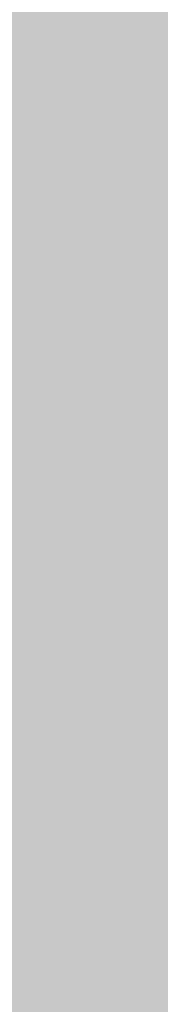
# Model space of a CAD drawing. Units: inches. Extents: x 2083 to 3317, y 1141 to 2115.
# Tile 172 of 256: x 3126.95594 to 3126.95825, y 1263.27402 to 1263.29018. Entities that reach past the tile are written whole.
import ezdxf

# ---------------------------------------------------------------- set-up
doc = ezdxf.new("R2010")
doc.units = ezdxf.units.IN
doc.layers.add('A-ANNO-DIMS', color=2, linetype='Continuous', lineweight=18)
doc.layers.add('A-WALL-PATT', color=251, linetype='Continuous', lineweight=13, true_color=0x636466)
doc.styles.get("Standard").update_dxf_attribs({"font": 'arial.ttf'})
doc.dimstyles.new('ISO-25', dxfattribs={"dimtxt": 12, "dimasz": 12, "dimexe": 1.25, "dimexo": 0.625, "dimtad": 1, "dimlunit": 3, "dimtxsty": 'Standard', "dimcen": 2.5, "dimadec": 0, "dimazin": 0, "dimtfac": 1, "dimtmove": 0, "dimatfit": 3, "dimfxl": 1, "dimarcsym": 0})

# ---------------------------------------------------------------- blocks, each defined once
blk = doc.blocks.new('*D26')
at = {"layer": 'A-ANNO-DIMS', "color": 0, "lineweight": -2, "transparency": 16777216}
for p, q in [((3088.985844, 1274.915092), (3088.985844, 1270.951963)), ((3111.240037, 1274.915092), (3111.240037, 1270.951963)), ((3076.985844, 1272.201963), (2840.262447, 1272.201963)), ((3111.240037, 1272.201963), (3088.985844, 1272.201963)), ((3123.240037, 1272.201963), (3135.240037, 1272.201963))]:
    blk.add_line(p, q, dxfattribs=at)
at = {"layer": 'A-ANNO-DIMS', "color": 0, "transparency": 16777216}
for points in [[(3076.985844, 1274.201963), (3076.985844, 1270.201963), (3088.985844, 1272.201963)], [(3123.240037, 1274.201963), (3123.240037, 1270.201963), (3111.240037, 1272.201963)]]:
    blk.add_solid(points, dxfattribs=at)
at = {"layer": 'Defpoints', "color": 0, "transparency": 16777216}
for p in [(3088.985844, 1275.540092), (3111.240037, 1275.540092), (3088.985844, 1272.201963)]:
    blk.add_point(p, dxfattribs=at)
at = {"layer": 'A-ANNO-DIMS', "color": 0, "transparency": 16777216, "insert": (2952.624146, 1279.031602), "char_height": 12, "attachment_point": 5}
blk.add_mtext('NIGHTSTAND 1\'-10 1/2" TYP.', dxfattribs=at)
blk = doc.blocks.new('*D27')
at = {"layer": 'A-ANNO-DIMS', "color": 0, "lineweight": -2, "transparency": 16777216}
for p, q in [((3114.578165, 1309.794285), (3114.578165, 1321.794285)), ((3111.865037, 1297.794285), (3115.828165, 1297.794285)), ((3114.578165, 1297.794285), (3114.578165, 1275.540092)), ((3111.865037, 1275.540092), (3115.828165, 1275.540092)), ((3114.578165, 1263.540092), (3114.578165, 1140.988591))]:
    blk.add_line(p, q, dxfattribs=at)
at = {"layer": 'A-ANNO-DIMS', "color": 0, "transparency": 16777216}
for points in [[(3112.578165, 1309.794285), (3116.578165, 1309.794285), (3114.578165, 1297.794285)], [(3112.578165, 1263.540092), (3116.578165, 1263.540092), (3114.578165, 1275.540092)]]:
    blk.add_solid(points, dxfattribs=at)
at = {"layer": 'Defpoints', "color": 0, "transparency": 16777216}
for p in [(3111.240037, 1297.794285), (3111.240037, 1275.540092), (3114.578165, 1275.540092)]:
    blk.add_point(p, dxfattribs=at)
at = {"layer": 'A-ANNO-DIMS', "color": 0, "transparency": 16777216, "insert": (3107.748527, 1196.264342), "char_height": 12, "attachment_point": 5, "rotation": 90}
blk.add_mtext('1\'-10 1/2" TYP.', dxfattribs=at)

msp = doc.modelspace()

# ---------------------------------------------------------------- hatches: boundary and pattern name
at = {"layer": 'A-WALL-PATT'}
h = msp.add_hatch(color=256, dxfattribs=at)
h.dxf.hatch_style = 1
h.paths.add_polyline_path([(3126.959783, 2020.76136), (2748.959783, 2020.76136), (2604.959783, 2020.76136), (2226.959783, 2020.76136), (2226.959783, 1702.76136), (2466.959783, 1702.76136), (2466.959783, 1582.76136), (2418.959783, 1582.76136), (2418.959783, 1477.76136), (2226.959783, 1477.76136), (2226.959783, 1263.26136), (2544.959783, 1263.26136), (2544.959783, 1411.76136), (2604.959783, 1411.76136), (2685.959783, 1411.76136), (2685.959783, 1420.76136), (2604.959783, 1420.76136), (2604.959783, 1573.76136), (2604.959783, 1702.76136), (2604.959783, 2011.76136), (2748.959783, 2011.76136), (2748.959783, 1702.76136), (2862.959783, 1702.76136), (2862.959783, 1621.76136), (2871.959783, 1621.76136), (2871.959783, 1702.76136), (2883.959783, 1702.76136), (2883.959783, 1706.939459, -0.026459), (2883.959783, 1711.76136), (2757.959783, 1711.76136), (2757.959783, 1807.76136), (2787.959783, 1807.76136), (2787.959783, 1812.26136), (2757.959783, 1812.26136), (2757.959783, 2011.76136), (2877.959783, 2011.76136), (2877.959783, 1812.26136), (2847.959783, 1812.26136), (2847.959783, 1807.76136), (2889.835742, 1807.76136), (2889.835742, 1812.26136), (2882.459783, 1812.26136), (2882.459783, 2011.76136), (3117.959783, 2011.76136), (3117.959783, 1812.26136), (2937.835742, 1812.26136), (2937.835742, 1807.76136), (2995.709783, 1807.76136), (2995.709783, 1796.117666), (3000.209783, 1796.117666), (3000.209783, 1807.76136), (3117.959783, 1807.76136), (3117.959783, 1711.76136), (3000.209783, 1711.76136), (3000.209783, 1760.117666), (2998.572705, 1760.117666, -0.020711), (2995.709783, 1760.117666), (2995.709783, 1711.76136), (2931.959783, 1711.76136), (2931.959783, 1702.76136), (3126.959783, 1702.76136)])
h.paths.add_polyline_path([(2471.459783, 2011.76136), (2471.459783, 1810.01136), (2462.716936, 1810.01136), (2462.716936, 1805.51136), (2505.959783, 1805.51136), (2505.959783, 1810.01136), (2475.959783, 1810.01136), (2475.959783, 2011.76136), (2595.959783, 2011.76136), (2595.959783, 1810.01136), (2565.959783, 1810.01136), (2565.959783, 1805.51136), (2595.959783, 1805.51136), (2595.959783, 1711.76136), (2235.959783, 1711.76136), (2235.959783, 1805.51136), (2353.709783, 1805.51136), (2353.709783, 1796.054162), (2358.209783, 1796.054162), (2358.209783, 1805.51136), (2414.716936, 1805.51136), (2414.716936, 1810.01136), (2235.959783, 1810.01136), (2235.959783, 2011.76136)], flags=16)
h.paths.add_polyline_path([(2270.204734, 1994.610008), (2270.204734, 1970.610008), (2246.204734, 1970.610008), (2246.204734, 1994.610008)], flags=0)
edge = h.paths.add_edge_path(flags=0)
edge.add_ellipse((2332.027391, 1899.798176), major_axis=(-3.042994, 3.042994), ratio=0.16825245, start_angle=-161.332166, end_angle=-156.307114, ccw=False)
edge.add_ellipse((2333.082037, 1898.74353), major_axis=(-1.054646, 1.054646), ratio=0.4535321, start_angle=-123.371019, end_angle=-94.159107)
edge = h.paths.add_edge_path(flags=0)
edge.add_ellipse((2332.027391, 1968.87629), major_axis=(3.042994, 3.042994), ratio=0.16825245, start_angle=18.667834, end_angle=23.692886)
edge.add_spline(control_points=[(2332.925596, 1970.691105), (2332.226768, 1970.3361), (2330.893709, 1969.658905), (2328.41308, 1970.932138), (2327.203934, 1967.748712), (2324.709596, 1969.955589), (2322.532822, 1967.012354), (2320.012846, 1971.295812), (2317.680308, 1968.157845), (2316.040526, 1967.102047), (2315.426904, 1966.809602)], knot_values=[0, 0, 0, 0, 2.267059, 4.324559, 6.685584, 8.878641, 11.121502, 14.300359, 17.755284, 19.732645, 19.732645, 19.732645, 19.732645], degree=3, periodic=0)
edge.add_ellipse((2332.027391, 1968.87629), major_axis=(3.042994, 3.042994), ratio=0.16825245, start_angle=18.667834, end_angle=23.692886, ccw=False)
edge.add_ellipse((2333.082037, 1969.930936), major_axis=(1.054646, 1.054646), ratio=0.4535321, start_angle=56.628981, end_angle=85.840893, ccw=False)
edge = h.paths.add_edge_path(flags=0)
edge.add_spline(control_points=[(2296.428287, 1967.987908), (2293.627804, 1965.336314), (2287.703624, 1959.727094), (2299.74386, 1949.995699), (2294.532591, 1935.668528), (2290.573228, 1920.603512), (2293.394124, 1909.973691), (2296.185407, 1904.966543)], knot_values=[0.099185, 0.099185, 0.099185, 0.099185, 0.345301, 0.619822, 0.982653, 1.386093, 1.810555, 1.810555, 1.810555, 1.810555], degree=3, periodic=0)
edge.add_spline(control_points=[(2296.185407, 1904.966543), (2297.383582, 1902.6193), (2298.000969, 1901.949312), (2298.55297, 1901.468155)], knot_values=[0.006246, 0.006246, 0.006246, 0.006246, 0.055476, 0.055476, 0.055476, 0.055476], degree=3, periodic=0)
edge.add_spline(control_points=[(2298.55297, 1901.468155), (2297.258612, 1900.923224), (2295.225294, 1900.232126), (2293.060229, 1900.614205), (2292.101423, 1900.788415), (2292.089578, 1900.790568)], knot_values=[0.312835, 0.312835, 0.312835, 0.312835, 0.40178, 0.474987, 0.475903, 0.475903, 0.475903, 0.475903], degree=3, periodic=0)
edge.add_arc((2292.793646, 1904.664109), 3.937008, 215.420897, 259.698179, ccw=False)
edge.add_spline(control_points=[(2289.585314, 1902.382304), (2289.476652, 1902.535087), (2289.36848, 1902.688035), (2289.260865, 1902.84117)], knot_values=[0.102872, 0.102872, 0.102872, 0.102872, 0.116896, 0.116896, 0.116896, 0.116896], degree=3, periodic=0)
edge.add_spline(control_points=[(2289.260865, 1902.84117), (2288.686604, 1902.550192), (2287.640048, 1902.019902), (2285.881337, 1901.873954), (2283.852972, 1901.504352), (2281.719987, 1899.710538), (2278.466991, 1899.492942), (2276.157136, 1901.883202), (2272.258953, 1899.804071), (2267.777605, 1901.843183), (2262.243882, 1900.184033), (2257.414927, 1901.782061), (2254.318374, 1900.72612), (2253.178285, 1900.337343)], knot_values=[0, 0, 0, 0, 1.907977, 3.477176, 5.261074, 7.972851, 11.680248, 13.717921, 16.939592, 22.789562, 27.502503, 33.595215, 37.145618, 37.145618, 37.145618, 37.145618], degree=3, periodic=0)
edge.add_line((2253.178285, 1900.337343), (2250.24424, 1902.84117))
edge.add_line((2250.24424, 1902.84117), (2250.24424, 1965.833296))
edge.add_line((2250.24424, 1965.833296), (2253.178285, 1968.337123))
edge.add_spline(control_points=[(2253.178285, 1968.337123), (2254.318374, 1967.948346), (2257.414927, 1966.892405), (2262.243882, 1968.490433), (2267.777605, 1966.831283), (2271.52673, 1968.537217), (2273.875914, 1967.828289), (2274.206701, 1967.727642)], knot_values=[0, 0, 0, 0, 0.09018, 0.244935, 0.364644, 0.513233, 0.537855, 0.537855, 0.537855, 0.537855], degree=3, periodic=0)
edge.add_arc((2274.352887, 1963.793349), 3.937008, 72.051134, 92.127949, ccw=False)
edge.add_arc((2281.296933, 1985.230003), 18.596298, 252.0511336, 288.5657217)
edge.add_arc((2292.316717, 1956.02888), 12.646081, 71.0267879, 113.7782184, ccw=False)
edge = h.paths.add_edge_path(flags=0)
edge.add_spline(control_points=[(2274.899415, 1951.856195), (2275.066156, 1951.616592), (2275.232687, 1951.376588), (2275.397987, 1951.135855)], knot_values=[1.409916, 1.409916, 1.409916, 1.409916, 1.43159, 1.43159, 1.43159, 1.43159], degree=3, periodic=0)
edge.add_spline(control_points=[(2275.397987, 1951.135855), (2275.792106, 1950.561885), (2276.179231, 1949.983774), (2276.545546, 1949.397103)], knot_values=[1.358238, 1.358238, 1.358238, 1.358238, 1.409916, 1.409916, 1.409916, 1.409916], degree=3, periodic=0)
edge.add_line((2276.545546, 1949.397103), (2277.437289, 1947.862185))
edge.add_spline(control_points=[(2277.437289, 1947.862185), (2276.303834, 1945.673115), (2274.639698, 1942.426882), (2274.631615, 1938.0939), (2272.799124, 1930.85155), (2274.356426, 1943.897046), (2275.947681, 1947.923356), (2276.545546, 1949.397103)], knot_values=[0.005632, 0.005632, 0.005632, 0.005632, 0.186014, 0.266002, 0.357087, 0.59639, 0.739732, 0.739732, 0.739732, 0.739732], degree=3, periodic=0)
edge.add_spline(control_points=[(2276.545546, 1949.397103), (2276.179231, 1949.983774), (2275.792106, 1950.561885), (2275.397987, 1951.135855)], knot_values=[1.358238, 1.358238, 1.358238, 1.358238, 1.409916, 1.409916, 1.409916, 1.409916], degree=3, periodic=0)
edge.add_spline(control_points=[(2275.397987, 1951.135855), (2274.9425, 1950.080452), (2274.20776, 1948.025272), (2273.934602, 1944.851477), (2272.468534, 1937.627489), (2273.466216, 1945.696466), (2274.700615, 1951.059472), (2274.899415, 1951.856195)], knot_values=[0.104364, 0.104364, 0.104364, 0.104364, 0.189636, 0.269624, 0.36071, 0.600013, 0.644622, 0.644622, 0.644622, 0.644622], degree=3, periodic=0)
h.paths.add_polyline_path([(2269.167514, 1963.127573, -0.357527), (2268.170633, 1960.97637, -0.092561), (2268.170633, 1939.436325, -0.357527), (2269.167514, 1937.285122, -0.357527), (2267.01631, 1938.282002, -0.164785), (2254.685581, 1938.282002, -0.357527), (2252.534378, 1937.285122, -0.357527), (2253.531259, 1939.436325, -0.092561), (2253.531259, 1960.97637, -0.357527), (2252.534378, 1963.127573, -0.357527), (2254.685581, 1962.130692, -0.164785), (2267.01631, 1962.130692, -0.357527)], flags=0)
h.paths.add_polyline_path([(2248.874068, 1967.8018), (2248.874068, 1957.02771), (2249.457783, 1957.02771), (2249.457783, 1911.646756), (2248.874068, 1911.646756), (2248.874068, 1900.872666), (2246.511863, 1900.872666, 0.197327), (2244.149658, 1902.456873), (2244.149658, 1966.217592, 0.197327), (2246.511863, 1967.8018)], flags=0)
h.paths.add_polyline_path([(2269.167514, 1931.389344, -0.357527), (2268.170633, 1929.238141, -0.092561), (2268.170633, 1907.698096, -0.357527), (2269.167514, 1905.546893, -0.357527), (2267.01631, 1906.543774, -0.164785), (2254.685581, 1906.543774, -0.357527), (2252.534378, 1905.546893, -0.357527), (2253.531259, 1907.698096, -0.092561), (2253.531259, 1929.238141, -0.357527), (2252.534378, 1931.389344, -0.357527), (2254.685581, 1930.392463, -0.164785), (2267.01631, 1930.392463, -0.357527)], flags=0)
edge = h.paths.add_edge_path(flags=0)
edge.add_spline(control_points=[(2276.196858, 1906.723702), (2276.168144, 1909.028928), (2276.114049, 1913.371852), (2270.598417, 1924.924978), (2273.905175, 1919.012779), (2275.921711, 1916.262063), (2275.47457, 1912.402149), (2277.257874, 1910.380621), (2276.696044, 1908.225036), (2276.646218, 1906.813023), (2276.617825, 1906.008407)], knot_values=[0, 0, 0, 0, 8.61026, 16.221274, 18.843057, 23.804898, 27.440828, 29.356102, 31.203478, 33.650687, 33.650687, 33.650687, 33.650687], degree=3, periodic=0)
edge.add_spline(control_points=[(2276.617825, 1906.008407), (2276.623313, 1905.624144), (2276.497738, 1904.628661), (2275.441779, 1903.854725), (2274.937314, 1903.08045), (2274.85908, 1902.84117)], knot_values=[0.156488, 0.156488, 0.156488, 0.156488, 0.184398, 0.231376, 0.250598, 0.250598, 0.250598, 0.250598], degree=3, periodic=0)
edge.add_line((2274.85908, 1902.84117), (2276.50598, 1902.84117))
edge.add_spline(control_points=[(2276.50598, 1902.84117), (2276.788308, 1903.08494), (2277.665071, 1904.125196), (2278.249538, 1904.340738), (2277.653872, 1908.527387), (2278.15567, 1906.227808), (2278.100464, 1905.285948), (2278.846675, 1904.069005), (2277.856785, 1903.414948), (2277.874191, 1902.99105), (2277.903562, 1902.84117)], knot_values=[0.059574, 0.059574, 0.059574, 0.059574, 0.080753, 0.103741, 0.16972, 0.176036, 0.207137, 0.240474, 0.262341, 0.27366, 0.27366, 0.27366, 0.27366], degree=3, periodic=0)
edge.add_line((2277.903562, 1902.84117), (2280.029825, 1902.84117))
edge.add_spline(control_points=[(2280.029825, 1902.84117), (2279.888221, 1903.088398), (2279.499257, 1903.981551), (2280.152284, 1905.939349), (2278.103615, 1909.657757), (2279.762395, 1907.185285), (2280.3279, 1904.874861), (2280.485109, 1903.48959), (2281.463269, 1903.249432), (2281.758343, 1902.936497), (2281.834036, 1902.84117)], knot_values=[0.013856, 0.013856, 0.013856, 0.013856, 0.034874, 0.088867, 0.107879, 0.126738, 0.158714, 0.193757, 0.217487, 0.226722, 0.226722, 0.226722, 0.226722], degree=3, periodic=0)
edge.add_spline(control_points=[(2281.834036, 1902.84117), (2281.787535, 1902.826703), (2281.647022, 1902.782988), (2281.395527, 1902.85949), (2281.088077, 1902.985242), (2280.720683, 1903.060902), (2280.333451, 1903.025726), (2280.124767, 1902.898879), (2280.029825, 1902.84117)], knot_values=[0, 0, 0, 0, 0.14413, 0.435517, 0.749276, 1.153046, 1.548371, 1.878348, 1.878348, 1.878348, 1.878348], degree=3, periodic=0)
edge.add_line((2280.029825, 1902.84117), (2277.903562, 1902.84117))
edge.add_spline(control_points=[(2277.903562, 1902.84117), (2277.892855, 1902.795855), (2277.865396, 1902.679637), (2277.607479, 1902.687483), (2277.27405, 1902.8007), (2276.837921, 1902.619775), (2276.583807, 1902.789261), (2276.50598, 1902.84117)], knot_values=[0, 0, 0, 0, 0.127189, 0.326199, 0.628009, 1.24357, 1.515331, 1.515331, 1.515331, 1.515331], degree=3, periodic=0)
edge.add_line((2276.50598, 1902.84117), (2274.85908, 1902.84117))
edge.add_spline(control_points=[(2274.85908, 1902.84117), (2274.814437, 1902.898587), (2274.72513, 1903.013446), (2274.493477, 1903.118968), (2274.244285, 1902.960539), (2273.937121, 1903.184942), (2273.614039, 1902.983143), (2273.408316, 1902.883045), (2273.322254, 1902.84117)], knot_values=[0, 0, 0, 0, 0.21843, 0.436957, 0.687977, 0.990379, 1.398396, 1.69185, 1.69185, 1.69185, 1.69185], degree=3, periodic=0)
edge.add_spline(control_points=[(2273.322254, 1902.84117), (2273.61674, 1903.445692), (2274.273998, 1904.538253), (2276.027239, 1904.573702), (2276.206963, 1906.583637), (2276.196858, 1906.723702)], knot_values=[0.012227, 0.012227, 0.012227, 0.012227, 0.059472, 0.106218, 0.134458, 0.134458, 0.134458, 0.134458], degree=3, periodic=0)
h.paths.add_polyline_path([(2270.776054, 1897.789828), (2270.776054, 1873.789828), (2246.776054, 1873.789828), (2246.776054, 1897.789828)], flags=0)
h.paths.add_polyline_path([(2353.709783, 1760.005059), (2353.709783, 1760.054162), (2358.209783, 1760.054162, -0.033729)], flags=0)
h.paths.add_polyline_path([(2321.819119, 1737.529186), (2341.995327, 1737.529186, -0.414214), (2343.203273, 1736.321241), (2343.203273, 1721.020596, -0.414214), (2341.995327, 1719.812651), (2321.819119, 1719.812651, -0.414214), (2320.611173, 1721.020596), (2320.611173, 1736.321241, -0.414214)], flags=0)
h.paths.add_polyline_path([(2324.23501, 1736.321241), (2339.579436, 1736.321241, -0.414214), (2341.995327, 1733.905349), (2341.995327, 1725.44973, -0.414214), (2339.579436, 1723.033839), (2333.680588, 1723.033839), (2333.845317, 1722.045467, -0.870646), (2335.425399, 1721.825893, -0.767327), (2333.922694, 1721.423245), (2331.291024, 1721.423245, -0.767327), (2329.788319, 1721.825893, -0.870646), (2331.368401, 1722.045467), (2331.53313, 1723.033839), (2324.23501, 1723.033839, -0.414214), (2321.819119, 1725.44973), (2321.819119, 1733.905349, -0.414214)], flags=0)
h.paths.add_polyline_path([(2570.483789, 1928.615444), (2589.683789, 1928.615444), (2590.168829, 1928.615444), (2590.168829, 1904.993397), (2570.483789, 1904.993397)], flags=0)
h.paths.add_polyline_path([(2574.447324, 1927.263822, -1), (2572.828836, 1927.263822, -1)], flags=0)
h.paths.add_polyline_path([(2573.089867, 1926.940877), (2573.925032, 1927.776042), (2574.147743, 1927.553332), (2573.312577, 1926.718166)], flags=0)
h.paths.add_polyline_path([(2578.779065, 1919.729618, -1), (2571.591663, 1919.729618, -1)], flags=0)
h.paths.add_polyline_path([(2578.385364, 1919.729618, -1), (2571.985364, 1919.729618, -1)], flags=0)
h.paths.add_polyline_path([(2331.595764, 1729.476216, -1), (2333.617954, 1729.476216, -1)], flags=0)
h.paths.add_polyline_path([(2578.034228, 1927.263822, -1), (2576.41574, 1927.263822, -1)], flags=0)
h.paths.add_polyline_path([(2576.688851, 1927.531089), (2576.911562, 1927.753799), (2577.746728, 1926.918634), (2577.524017, 1926.695923)], flags=0)
h.paths.add_polyline_path([(2578.139065, 1909.859539, -1), (2572.231663, 1909.859539, -1)], flags=0)
h.paths.add_polyline_path([(2577.745364, 1909.859539, -1), (2572.625364, 1909.859539, -1)], flags=0)
h.paths.add_polyline_path([(2583.797718, 1927.263822, -1), (2582.179229, 1927.263822, -1)], flags=0)
h.paths.add_polyline_path([(2582.718649, 1927.753799), (2583.553814, 1926.918634), (2583.331103, 1926.695923), (2582.495938, 1927.531089)], flags=0)
h.paths.add_polyline_path([(2582.495938, 1927.531089), (2582.718649, 1927.753799), (2583.553814, 1926.918634), (2583.331103, 1926.695923)], flags=0)
h.paths.add_polyline_path([(2587.739065, 1920.529618, -1), (2581.831663, 1920.529618, -1)], flags=0)
h.paths.add_polyline_path([(2587.345364, 1920.529618, -1), (2582.225364, 1920.529618, -1)], flags=0)
h.paths.add_polyline_path([(2587.384622, 1927.263822, -1), (2585.766133, 1927.263822, -1)], flags=0)
h.paths.add_polyline_path([(2586.081993, 1926.980247), (2586.917158, 1927.815412), (2587.139869, 1927.592702), (2586.304703, 1926.757536)], flags=0)
h.paths.add_polyline_path([(2588.379065, 1910.659539, -1), (2581.191663, 1910.659539, -1)], flags=0)
h.paths.add_polyline_path([(2587.985364, 1910.659539, -1), (2581.585364, 1910.659539, -1)], flags=0)
h.paths.add_polyline_path([(2417.167729, 1729.477895), (2437.343937, 1729.477895, -0.414214), (2438.551883, 1728.26995), (2438.551883, 1712.969306, -0.414214), (2437.343937, 1711.76136), (2417.167729, 1711.76136, -0.414214), (2415.959783, 1712.969306), (2415.959783, 1728.26995, -0.414214)], flags=0)
h.paths.add_polyline_path([(2419.58362, 1728.26995), (2434.928046, 1728.26995, -0.414214), (2437.343937, 1725.854059), (2437.343937, 1717.39844, -0.414214), (2434.928046, 1714.982548), (2429.029199, 1714.982548), (2429.193927, 1713.994176, -0.870646), (2430.774009, 1713.774603, -0.767327), (2429.271304, 1713.371954), (2426.639634, 1713.371954, -0.767327), (2425.136929, 1713.774603, -0.870646), (2426.717011, 1713.994176), (2426.88174, 1714.982548), (2419.58362, 1714.982548, -0.414214), (2417.167729, 1717.39844), (2417.167729, 1725.854059, -0.414214)], flags=0)
h.paths.add_polyline_path([(2419.58362, 1728.26995), (2434.928046, 1728.26995, -0.414214), (2437.343937, 1725.854059), (2437.343937, 1717.39844, -0.414214), (2434.928046, 1714.982548), (2429.029199, 1714.982548), (2428.358118, 1719.009034), (2427.552821, 1719.009034), (2426.88174, 1714.982548), (2419.58362, 1714.982548, -0.414214), (2417.167729, 1717.39844), (2417.167729, 1725.854059, -0.414214)], flags=0)
h.paths.add_polyline_path([(2426.944374, 1721.424925, -1), (2428.966564, 1721.424925, -1)], flags=0)
h.paths.add_polyline_path([(2475.959783, 1702.76136), (2595.959783, 1702.76136), (2595.959783, 1582.76136), (2475.959783, 1582.76136)], flags=16)
h.paths.add_polyline_path([(2427.959783, 1573.76136), (2595.959783, 1573.76136), (2595.959783, 1468.76136), (2595.959783, 1420.76136), (2384.459783, 1420.76136), (2384.459783, 1468.76136), (2427.959783, 1468.76136)], flags=16)
h.paths.add_polyline_path([(2379.959783, 1468.76136), (2379.959783, 1420.76136), (2235.959783, 1420.76136), (2235.959783, 1468.76136)], flags=16)
h.paths.add_polyline_path([(2317.815996, 1466.695767), (2337.992205, 1466.695767, -0.414214), (2339.20015, 1465.487821), (2339.20015, 1450.187177, -0.414214), (2337.992205, 1448.979232), (2317.815996, 1448.979232, -0.414214), (2316.608051, 1450.187177), (2316.608051, 1465.487821, -0.414214)], flags=0)
h.paths.add_polyline_path([(2320.231887, 1465.487821), (2335.576313, 1465.487821, -0.414214), (2337.992205, 1463.07193), (2337.992205, 1454.616311, -0.414214), (2335.576313, 1452.20042), (2329.677466, 1452.20042), (2329.842195, 1451.212047, -0.870646), (2331.422276, 1450.992474, -0.767327), (2329.919571, 1450.589826), (2327.287902, 1450.589826, -0.767327), (2325.785197, 1450.992474, -0.870646), (2327.365278, 1451.212047), (2327.530007, 1452.20042), (2320.231887, 1452.20042, -0.414214), (2317.815996, 1454.616311), (2317.815996, 1463.07193, -0.414214)], flags=0)
h.paths.add_polyline_path([(2320.231887, 1465.487821), (2335.576313, 1465.487821, -0.414214), (2337.992205, 1463.07193), (2337.992205, 1454.616311, -0.414214), (2335.576313, 1452.20042), (2329.677466, 1452.20042), (2329.006385, 1456.226905), (2328.201088, 1456.226905), (2327.530007, 1452.20042), (2320.231887, 1452.20042, -0.414214), (2317.815996, 1454.616311), (2317.815996, 1463.07193, -0.414214)], flags=0)
h.paths.add_polyline_path([(2327.592641, 1458.642796, -1), (2329.614832, 1458.642796, -1)], flags=0)
h.paths.add_polyline_path([(2244.411744, 1433.340453), (2241.920945, 1433.340453, -0.414214), (2240.017856, 1435.243542), (2240.017856, 1440.952808, -0.414211), (2241.920925, 1442.855897), (2244.411744, 1442.855897, -1.976472)], flags=0)
h.paths.add_polyline_path([(2245.356888, 1434.397536, -0.414214), (2245.356888, 1441.798814, -2.144098)], flags=0)
h.paths.add_polyline_path([(2535.959783, 1416.26136), (2535.959783, 1272.26136), (2235.959783, 1272.26136), (2235.959783, 1416.26136)], flags=16)
h.paths.add_polyline_path([(2260.119561, 1384.292841), (2260.119561, 1362.038649), (2237.865369, 1362.038649), (2237.865369, 1384.292841)], flags=0)
edge = h.paths.add_edge_path(flags=0)
edge.add_line((2318.251847, 1362.093298), (2318.145797, 1362.000973))
edge.add_ellipse((2317.445116, 1360.431044), major_axis=(2.82164, 2.82164), ratio=0.16825245, start_angle=18.667834, end_angle=20.948127, ccw=False)
edge.add_ellipse((2318.423045, 1361.408974), major_axis=(0.977929, 0.977929), ratio=0.4535321, start_angle=56.628981, end_angle=70.226201, ccw=False)
edge = h.paths.add_edge_path(flags=0)
edge.add_line((2319.10737, 1295.571078), (2319.015044, 1295.677128))
edge.add_ellipse((2317.445116, 1296.377809), major_axis=(-2.82164, 2.82164), ratio=0.16825245, start_angle=-161.332166, end_angle=-159.051873, ccw=False)
edge.add_ellipse((2318.423045, 1295.39988), major_axis=(-0.977929, 0.977929), ratio=0.4535321, start_angle=-123.371019, end_angle=-109.773799)
edge = h.paths.add_edge_path(flags=0)
edge.add_spline(control_points=[(2284.210349, 1301.170219), (2284.580688, 1300.444719), (2284.891189, 1299.892024), (2285.159553, 1299.461018)], knot_values=[0.039066, 0.039066, 0.039066, 0.039066, 0.055476, 0.055476, 0.055476, 0.055476], degree=3, periodic=0)
edge.add_line((2285.159553, 1299.461018), (2284.210349, 1301.170219))
edge = h.paths.add_edge_path(flags=0)
edge.add_line((2280.412458, 1297.298013), (2283.369991, 1297.036122))
edge.add_line((2283.369991, 1297.036122), (2286.40569, 1297.92631))
edge.add_spline(control_points=[(2286.40569, 1297.92631), (2285.305487, 1297.463119), (2284.344777, 1297.129151), (2283.369991, 1297.036122)], knot_values=[0.394369, 0.394369, 0.394369, 0.394369, 0.475903, 0.475903, 0.475903, 0.475903], degree=3, periodic=0)
edge.add_spline(control_points=[(2283.369991, 1297.036122), (2283.28139, 1297.027666), (2282.316289, 1296.957336), (2281.312502, 1297.134479), (2280.423441, 1297.296016), (2280.412458, 1297.298013)], knot_values=[0.312835, 0.312835, 0.312835, 0.312835, 0.320246, 0.393453, 0.394369, 0.394369, 0.394369, 0.394369], degree=3, periodic=0)
edge = h.paths.add_edge_path(flags=0)
edge.add_line((2284.435561, 1359.607285), (2280.446291, 1355.328047))
edge.add_line((2280.446291, 1355.328047), (2279.579987, 1351.017754))
edge.add_line((2279.579987, 1351.017754), (2282.412974, 1346.580433))
edge.add_spline(control_points=[(2282.412974, 1346.580433), (2283.153331, 1345.589236), (2284.252896, 1344.028897), (2284.801037, 1342.387167), (2284.935162, 1341.805544)], knot_values=[1.240098, 1.240098, 1.240098, 1.240098, 1.332892, 1.382712, 1.382712, 1.382712, 1.382712], degree=3, periodic=0)
edge.add_spline(control_points=[(2284.935162, 1341.805544), (2285.319108, 1340.1406), (2285.233029, 1338.409204), (2284.909938, 1336.654122)], knot_values=[1.097484, 1.097484, 1.097484, 1.097484, 1.240098, 1.240098, 1.240098, 1.240098], degree=3, periodic=0)
edge.add_spline(control_points=[(2284.909938, 1336.654122), (2284.586848, 1334.89904), (2284.026745, 1333.120272), (2283.462644, 1331.360585)], knot_values=[0.95487, 0.95487, 0.95487, 0.95487, 1.097484, 1.097484, 1.097484, 1.097484], degree=3, periodic=0)
edge.add_line((2283.462644, 1331.360585), (2281.890376, 1326.153357))
edge.add_line((2281.890376, 1326.153357), (2280.756259, 1321.056089))
edge.add_line((2280.756259, 1321.056089), (2280.299205, 1316.001977))
edge.add_line((2280.299205, 1316.001977), (2280.715933, 1310.950068))
edge.add_line((2280.715933, 1310.950068), (2282.028094, 1305.972137))
edge.add_line((2282.028094, 1305.972137), (2284.210349, 1301.170219))
edge.add_spline(control_points=[(2284.210349, 1301.170219), (2283.340731, 1302.730185), (2282.611904, 1304.336493), (2282.028094, 1305.972137)], knot_values=[0.099185, 0.099185, 0.099185, 0.099185, 0.241799, 0.241799, 0.241799, 0.241799], degree=3, periodic=0)
edge.add_spline(control_points=[(2282.028094, 1305.972137), (2281.444283, 1307.60778), (2281.005489, 1309.272759), (2280.715933, 1310.950068)], knot_values=[0.241799, 0.241799, 0.241799, 0.241799, 0.384413, 0.384413, 0.384413, 0.384413], degree=3, periodic=0)
edge.add_spline(control_points=[(2280.715933, 1310.950068), (2280.433241, 1312.587613), (2280.289386, 1314.276959), (2280.298894, 1315.962032), (2280.299205, 1316.001977)], knot_values=[0.384413, 0.384413, 0.384413, 0.384413, 0.523647, 0.527028, 0.527028, 0.527028, 0.527028], degree=3, periodic=0)
edge.add_spline(control_points=[(2280.299205, 1316.001977), (2280.312326, 1317.686955), (2280.477871, 1319.367926), (2280.756259, 1321.056089)], knot_values=[0.527028, 0.527028, 0.527028, 0.527028, 0.669642, 0.669642, 0.669642, 0.669642], degree=3, periodic=0)
edge.add_spline(control_points=[(2280.756259, 1321.056089), (2281.034648, 1322.744252), (2281.42588, 1324.439608), (2281.890376, 1326.153357)], knot_values=[0.669642, 0.669642, 0.669642, 0.669642, 0.812256, 0.812256, 0.812256, 0.812256], degree=3, periodic=0)
edge.add_spline(control_points=[(2281.890376, 1326.153357), (2282.264383, 1327.533251), (2282.78787, 1329.26181), (2283.352751, 1331.01778), (2283.462644, 1331.360585)], knot_values=[0.812256, 0.812256, 0.812256, 0.812256, 0.927087, 0.95487, 0.95487, 0.95487, 0.95487], degree=3, periodic=0)
edge.add_line((2283.462644, 1331.360585), (2284.909938, 1336.654122))
edge.add_line((2284.909938, 1336.654122), (2284.935162, 1341.805544))
edge.add_line((2284.935162, 1341.805544), (2282.412974, 1346.580433))
edge.add_spline(control_points=[(2282.412974, 1346.580433), (2281.275127, 1348.103792), (2280.078447, 1349.570318), (2279.579987, 1351.017754)], knot_values=[1.382712, 1.382712, 1.382712, 1.382712, 1.525326, 1.525326, 1.525326, 1.525326], degree=3, periodic=0)
edge.add_spline(control_points=[(2279.579987, 1351.017754), (2279.443282, 1351.414721), (2279.136312, 1352.856922), (2279.73519, 1354.290385), (2280.446291, 1355.328047)], knot_values=[1.525326, 1.525326, 1.525326, 1.525326, 1.564439, 1.667941, 1.667941, 1.667941, 1.667941], degree=3, periodic=0)
edge.add_spline(control_points=[(2280.446291, 1355.328047), (2281.426113, 1356.757835), (2282.930837, 1358.18256), (2284.435561, 1359.607285)], knot_values=[1.667941, 1.667941, 1.667941, 1.667941, 1.810555, 1.810555, 1.810555, 1.810555], degree=3, periodic=0)
edge.add_arc((2280.623075, 1348.518181), 11.72618, 71.0267879, 113.7782184)
edge.add_arc((2270.404892, 1375.595156), 17.243567, 252.0511336, 288.5657217, ccw=False)
edge.add_arc((2263.965969, 1355.717847), 3.650622, 72.051134, 92.127949)
edge.add_arc((2263.965969, 1355.717847), 3.650622, 92.127949, 177.98513)
edge.add_spline(control_points=[(2260.317604, 1355.846199), (2260.260417, 1354.220668), (2260.551278, 1350.186547), (2262.999344, 1346.766251), (2264.472741, 1344.649024)], knot_values=[1.43159, 1.43159, 1.43159, 1.43159, 1.564144, 1.770695, 1.770695, 1.770695, 1.770695], degree=3, periodic=0)
edge.add_line((2264.472741, 1344.649024), (2264.93559, 1343.98253))
edge.add_spline(control_points=[(2263.801044, 1340.248105), (2263.843238, 1340.514088), (2264.067244, 1341.756465), (2264.512693, 1343.002453), (2264.935047, 1343.981083)], knot_values=[0.53657, 0.53657, 0.53657, 0.53657, 0.559349, 0.644622, 0.644622, 0.644622, 0.644622], degree=3, periodic=0)
edge.add_spline(control_points=[(2264.935047, 1343.981083), (2265.117771, 1343.714975), (2265.298875, 1343.447906), (2265.476756, 1343.179365)], knot_values=[1.384077, 1.384077, 1.384077, 1.384077, 1.409916, 1.409916, 1.409916, 1.409916], degree=3, periodic=0)
edge.add_spline(control_points=[(2265.476756, 1343.179365), (2265.654637, 1342.910823), (2265.829296, 1342.64081), (2265.99913, 1342.368812)], knot_values=[1.358238, 1.358238, 1.358238, 1.358238, 1.384077, 1.384077, 1.384077, 1.384077], degree=3, periodic=0)
edge.add_line((2265.99913, 1342.368812), (2266.826006, 1340.945547))
edge.add_spline(control_points=[(2266.826006, 1340.945547), (2268.894401, 1337.089691), (2271.398173, 1325.843001), (2270.516164, 1310.568557), (2275.919376, 1301.860609), (2277.789511, 1299.19945)], knot_values=[0.116896, 0.116896, 0.116896, 0.116896, 0.472987, 1.050969, 1.313793, 1.313793, 1.313793, 1.313793], degree=3, periodic=0)
edge.add_spline(control_points=[(2277.789511, 1299.19945), (2277.839405, 1299.128452), (2277.889428, 1299.057498), (2277.939572, 1298.986584)], knot_values=[0.109884, 0.109884, 0.109884, 0.109884, 0.116896, 0.116896, 0.116896, 0.116896], degree=3, periodic=0)
edge.add_line((2277.939572, 1298.986584), (2277.788849, 1299.199114))
edge.add_spline(control_points=[(2277.788849, 1299.199114), (2277.256582, 1298.929414), (2276.28635, 1298.437902), (2275.039352, 1298.334419), (2274.38333, 1298.238895), (2274.215254, 1298.209338)], knot_values=[33.12187, 33.12187, 33.12187, 33.12187, 35.029056, 36.598255, 37.144827, 37.144827, 37.144827, 37.144827], degree=3, periodic=0)
edge.add_line((2274.215254, 1298.209338), (2273.073147, 1297.892961))
edge.add_spline(control_points=[(2273.073147, 1297.892961), (2272.322936, 1297.579784), (2271.039151, 1296.510508), (2269.248395, 1296.226062), (2268.4231, 1296.374654)], knot_values=[26.532584, 26.532584, 26.532584, 26.532584, 29.198919, 31.839101, 31.839101, 31.839101, 31.839101], degree=3, periodic=0)
edge.add_line((2268.4231, 1296.374654), (2263.878501, 1297.457534))
edge.add_spline(control_points=[(2263.878501, 1297.457534), (2263.556077, 1297.359435), (2261.860306, 1296.838694), (2260.23878, 1297.282407), (2258.933454, 1297.516461)], knot_values=[15.919551, 15.919551, 15.919551, 15.919551, 16.939592, 21.226067, 21.226067, 21.226067, 21.226067], degree=3, periodic=0)
edge.add_line((2258.933454, 1297.516461), (2254.055233, 1297.32901))
edge.add_spline(control_points=[(2254.055233, 1297.32901), (2253.755525, 1297.295815), (2252.113683, 1297.165174), (2250.461869, 1297.544221), (2249.129686, 1297.667882)], knot_values=[5.306517, 5.306517, 5.306517, 5.306517, 6.276435, 10.613034, 10.613034, 10.613034, 10.613034], degree=3, periodic=0)
edge.add_line((2249.129686, 1297.667882), (2244.33165, 1296.877756))
edge.add_line((2244.33165, 1296.877756), (2241.611033, 1299.19945))
edge.add_line((2241.611033, 1299.19945), (2241.611033, 1357.609404))
edge.add_line((2241.611033, 1357.609404), (2244.33165, 1359.931097))
edge.add_line((2244.33165, 1359.931097), (2252.728823, 1359.542692))
edge.add_spline(control_points=[(2252.728823, 1359.542692), (2252.870939, 1359.54644), (2253.30574, 1359.548172), (2253.739845, 1359.514274), (2254.031742, 1359.482426)], knot_values=[0.233291, 0.233291, 0.233291, 0.233291, 0.244935, 0.268927, 0.268927, 0.268927, 0.268927], degree=3, periodic=0)
edge.add_line((2254.031742, 1359.482426), (2259.58719, 1359.41639))
edge.add_spline(control_points=[(2259.58719, 1359.41639), (2260.677068, 1359.628503), (2262.073197, 1359.897003), (2263.523692, 1359.459278), (2263.830417, 1359.365952)], knot_values=[0.422516, 0.422516, 0.422516, 0.422516, 0.513233, 0.537855, 0.537855, 0.537855, 0.537855], degree=3, periodic=0)
edge.add_arc((2263.965969, 1355.717847), 3.650622, 72.051134, 92.127949, ccw=False)
edge.add_arc((2270.404892, 1375.595156), 17.243567, 252.0511336, 288.5657217)
edge.add_arc((2280.623075, 1348.518181), 11.72618, 71.0267879, 113.7782184, ccw=False)
h.paths.add_polyline_path([(2240.34053, 1359.434715), (2240.34053, 1349.444353), (2240.881785, 1349.444353), (2240.881785, 1307.3645), (2240.34053, 1307.3645), (2240.34053, 1297.374138), (2238.150157, 1297.374138, 0.197327), (2235.959783, 1298.843108), (2235.959783, 1357.965746, 0.197327), (2238.150157, 1359.434715)], flags=0)
h.paths.add_polyline_path([(2259.15779, 1355.1005, -0.357527), (2258.233425, 1353.10578, -0.092561), (2258.233425, 1333.132601, -0.357527), (2259.15779, 1331.13788, -0.357527), (2257.16307, 1332.062246, -0.164785), (2245.729302, 1332.062246, -0.357527), (2243.734582, 1331.13788, -0.357527), (2244.658947, 1333.132601, -0.092561), (2244.658947, 1353.10578, -0.357527), (2243.734582, 1355.1005, -0.357527), (2245.729302, 1354.176135, -0.164785), (2257.16307, 1354.176135, -0.357527)], flags=0)
edge = h.paths.add_edge_path(flags=0)
edge.add_line((2265.99913, 1342.368812), (2266.826006, 1340.945547))
edge.add_line((2266.826006, 1340.945547), (2265.307557, 1337.814066))
edge.add_line((2265.307557, 1337.814066), (2264.358232, 1334.652939))
edge.add_line((2264.358232, 1334.652939), (2264.262012, 1333.799705))
edge.add_spline(control_points=[(2264.262012, 1333.799705), (2264.208357, 1333.187055), (2264.16206, 1332.365525), (2264.007144, 1331.413933), (2263.969049, 1331.201834)], knot_values=[0.464444, 0.464444, 0.464444, 0.464444, 0.516691, 0.531608, 0.531608, 0.531608, 0.531608], degree=3, periodic=0)
edge.add_spline(control_points=[(2263.969049, 1331.201834), (2263.774535, 1330.118873), (2263.42437, 1328.790839), (2263.25742, 1328.530652), (2263.234028, 1328.514612)], knot_values=[0.372682, 0.372682, 0.372682, 0.372682, 0.44885, 0.464444, 0.464444, 0.464444, 0.464444], degree=3, periodic=0)
edge.add_spline(control_points=[(2263.234028, 1328.514612), (2263.096382, 1328.420227), (2263.13117, 1329.301477), (2263.274953, 1330.615749)], knot_values=[0.280919, 0.280919, 0.280919, 0.280919, 0.372682, 0.372682, 0.372682, 0.372682], degree=3, periodic=0)
edge.add_spline(control_points=[(2263.274953, 1330.615749), (2263.418736, 1331.930022), (2263.671515, 1333.677318), (2263.969852, 1335.315027)], knot_values=[0.189157, 0.189157, 0.189157, 0.189157, 0.280919, 0.280919, 0.280919, 0.280919], degree=3, periodic=0)
edge.add_spline(control_points=[(2263.969852, 1335.315027), (2264.100496, 1336.032192), (2264.418783, 1337.621911), (2264.754848, 1338.86443), (2264.947419, 1339.491124)], knot_values=[0.097394, 0.097394, 0.097394, 0.097394, 0.137578, 0.189157, 0.189157, 0.189157, 0.189157], degree=3, periodic=0)
edge.add_spline(control_points=[(2264.947419, 1339.491124), (2265.290017, 1340.606055), (2265.644238, 1341.493996), (2265.99913, 1342.368812)], knot_values=[0.005632, 0.005632, 0.005632, 0.005632, 0.097394, 0.097394, 0.097394, 0.097394], degree=3, periodic=0)
h.paths.add_polyline_path([(2259.15779, 1325.670973, -0.357527), (2258.233425, 1323.676253, -0.092561), (2258.233425, 1303.703073, -0.357527), (2259.15779, 1301.708353, -0.357527), (2257.16307, 1302.632719, -0.164785), (2245.729302, 1302.632719, -0.357527), (2243.734582, 1301.708353, -0.357527), (2244.658947, 1303.703073, -0.092561), (2244.658947, 1323.676253, -0.357527), (2243.734582, 1325.670973, -0.357527), (2245.729302, 1324.746608, -0.164785), (2257.16307, 1324.746608, -0.357527)], flags=0)
edge = h.paths.add_edge_path(flags=0)
edge.add_spline(control_points=[(2261.708938, 1317.311421), (2261.679482, 1317.41758), (2261.761858, 1317.388535), (2262.490736, 1316.089873), (2262.962185, 1315.300897)], knot_values=[14.955861, 14.955861, 14.955861, 14.955861, 16.221274, 18.694826, 18.694826, 18.694826, 18.694826], degree=3, periodic=0)
edge.add_spline(control_points=[(2262.962185, 1315.300897), (2262.990437, 1315.253617), (2263.702096, 1314.067376), (2264.348983, 1313.127153), (2264.730054, 1312.164154)], knot_values=[18.694826, 18.694826, 18.694826, 18.694826, 18.843057, 22.433791, 22.433791, 22.433791, 22.433791], degree=3, periodic=0)
edge.add_spline(control_points=[(2264.730054, 1312.164154), (2264.875565, 1311.796437), (2265.176873, 1310.769807), (2265.143069, 1309.559262), (2265.247736, 1308.824193)], knot_values=[22.433791, 22.433791, 22.433791, 22.433791, 23.804898, 26.172756, 26.172756, 26.172756, 26.172756], degree=3, periodic=0)
edge.add_line((2265.247736, 1308.824193), (2265.850774, 1307.171888))
edge.add_spline(control_points=[(2265.850774, 1307.171888), (2266.065025, 1306.821678), (2266.384387, 1306.332246), (2266.4244, 1305.780549), (2266.420369, 1305.611216)], knot_values=[28.062562, 28.062562, 28.062562, 28.062562, 29.356102, 29.911721, 29.911721, 29.911721, 29.911721], degree=3, periodic=0)
edge.add_spline(control_points=[(2266.420369, 1305.611216), (2266.416116, 1305.43259), (2266.393999, 1305.249998), (2266.364777, 1305.065857)], knot_values=[29.911721, 29.911721, 29.911721, 29.911721, 30.497837, 30.497837, 30.497837, 30.497837], degree=3, periodic=0)
edge.add_line((2266.364777, 1305.065857), (2266.066151, 1302.136295))
edge.add_spline(control_points=[(2266.066151, 1302.136295), (2266.07124, 1301.779984), (2265.998076, 1301.199985), (2265.663266, 1300.758961), (2265.508908, 1300.585882)], knot_values=[0.156488, 0.156488, 0.156488, 0.156488, 0.184398, 0.203543, 0.203543, 0.203543, 0.203543], degree=3, periodic=0)
edge.add_line((2265.508908, 1300.585882), (2264.435341, 1299.19945))
edge.add_line((2264.435341, 1299.19945), (2265.962442, 1299.19945))
edge.add_line((2265.962442, 1299.19945), (2267.33599, 1301.175276))
edge.add_line((2267.33599, 1301.175276), (2267.311667, 1301.986237))
edge.add_spline(control_points=[(2267.311667, 1301.986237), (2267.261111, 1302.862396), (2267.160212, 1303.737132), (2267.271486, 1303.325896)], knot_values=[0.126229, 0.126229, 0.126229, 0.126229, 0.166617, 0.166617, 0.166617, 0.166617], degree=3, periodic=0)
edge.add_spline(control_points=[(2267.271486, 1303.325896), (2267.280035, 1303.294305), (2267.309785, 1303.175366), (2267.37345, 1302.883608), (2267.406123, 1302.682829), (2267.417926, 1302.601025)], knot_values=[0.166617, 0.166617, 0.166617, 0.166617, 0.16972, 0.176036, 0.180765, 0.180765, 0.180765, 0.180765], degree=3, periodic=0)
edge.add_spline(control_points=[(2267.743891, 1300.987505), (2267.687583, 1301.150943), (2267.48052, 1301.656664), (2267.483751, 1302.144788), (2267.417926, 1302.601025)], knot_values=[0.180765, 0.180765, 0.180765, 0.180765, 0.193767, 0.220139, 0.220139, 0.220139, 0.220139], degree=3, periodic=0)
edge.add_line((2267.417926, 1302.601025), (2267.743891, 1300.987505))
edge.add_spline(control_points=[(2267.743891, 1300.987505), (2267.831961, 1300.731878), (2267.932021, 1300.309904), (2267.554841, 1299.974518), (2267.429366, 1299.829207)], knot_values=[0.220139, 0.220139, 0.220139, 0.220139, 0.240474, 0.25489, 0.25489, 0.25489, 0.25489], degree=3, periodic=0)
edge.add_line((2267.429366, 1299.829207), (2267.258361, 1299.19945))
edge.add_line((2267.258361, 1299.19945), (2269.229956, 1299.19945))
edge.add_spline(control_points=[(2269.229956, 1299.19945), (2269.098653, 1299.428694), (2268.842774, 1300.016251), (2269.011575, 1300.915923), (2268.946796, 1301.66074)], knot_values=[0.013856, 0.013856, 0.013856, 0.013856, 0.034874, 0.067073, 0.067073, 0.067073, 0.067073], degree=3, periodic=0)
edge.add_line((2268.946796, 1301.66074), (2268.431582, 1303.603109))
edge.add_spline(control_points=[(2268.431582, 1303.603109), (2268.175596, 1304.192375), (2267.596214, 1305.251298), (2268.040698, 1304.62321), (2268.251394, 1304.282421)], knot_values=[0.090155, 0.090155, 0.090155, 0.090155, 0.107879, 0.120289, 0.120289, 0.120289, 0.120289], degree=3, periodic=0)
edge.add_spline(control_points=[(2268.251394, 1304.282421), (2268.360882, 1304.105329), (2269.057753, 1302.917983), (2269.382691, 1301.590419), (2269.521405, 1300.775931), (2269.57522, 1300.555784)], knot_values=[0.120289, 0.120289, 0.120289, 0.120289, 0.126738, 0.158714, 0.173506, 0.173506, 0.173506, 0.173506], degree=3, periodic=0)
edge.add_line((2269.57522, 1300.555784), (2270.685798, 1299.421258))
edge.add_spline(control_points=[(2270.685798, 1299.421258), (2270.767221, 1299.357251), (2270.837852, 1299.281401), (2270.902925, 1299.19945)], knot_values=[0.21816, 0.21816, 0.21816, 0.21816, 0.226722, 0.226722, 0.226722, 0.226722], degree=3, periodic=0)
edge.add_line((2270.937201, 1299.192913), (2270.902925, 1299.19945))
edge.add_spline(control_points=[(2270.902925, 1299.19945), (2270.859806, 1299.186035), (2270.729515, 1299.1455), (2270.496314, 1299.216437), (2270.271661, 1299.308323), (2270.121017, 1299.347961), (2270.063339, 1299.359557)], knot_values=[0.939174, 0.939174, 0.939174, 0.939174, 1.083304, 1.374691, 1.68845, 1.878348, 1.878348, 1.878348, 1.878348], degree=3, periodic=0)
edge.add_line((2270.063339, 1299.359557), (2269.229956, 1299.19945))
edge.add_line((2269.229956, 1299.19945), (2267.258361, 1299.19945))
edge.add_spline(control_points=[(2267.258361, 1299.19945), (2267.248433, 1299.157431), (2267.222971, 1299.049667), (2266.983816, 1299.056942), (2266.80921, 1299.11623), (2266.676905, 1299.109091), (2266.636531, 1299.104815)], knot_values=[0.757665, 0.757665, 0.757665, 0.757665, 0.884854, 1.083864, 1.385675, 1.515331, 1.515331, 1.515331, 1.515331], degree=3, periodic=0)
edge.add_spline(control_points=[(2266.636531, 1299.104815), (2266.485225, 1299.088788), (2266.235807, 1299.017123), (2266.034608, 1299.151317), (2265.962442, 1299.19945)], knot_values=[0, 0, 0, 0, 0.485905, 0.757665, 0.757665, 0.757665, 0.757665], degree=3, periodic=0)
edge.add_line((2265.962442, 1299.19945), (2264.435341, 1299.19945))
edge.add_line((2264.435341, 1299.19945), (2263.858444, 1299.367118))
edge.add_spline(control_points=[(2263.858444, 1299.367118), (2263.818943, 1299.370905), (2263.779528, 1299.385721), (2263.740131, 1299.401504)], knot_values=[0.845925, 0.845925, 0.845925, 0.845925, 0.978627, 0.978627, 0.978627, 0.978627], degree=3, periodic=0)
edge.add_line((2263.721786, 1299.396425), (2263.010306, 1299.19945))
edge.add_spline(control_points=[(2263.010306, 1299.19945), (2263.245794, 1299.682859), (2263.506032, 1300.128107), (2263.873494, 1300.408028)], knot_values=[0.012227, 0.012227, 0.012227, 0.012227, 0.052971, 0.052971, 0.052971, 0.052971], degree=3, periodic=0)
edge.add_spline(control_points=[(2263.873494, 1300.408028), (2263.932131, 1300.452695), (2264.084243, 1300.552979), (2264.255189, 1300.624223), (2264.359686, 1300.664747)], knot_values=[0.052971, 0.052971, 0.052971, 0.052971, 0.059472, 0.069086, 0.069086, 0.069086, 0.069086], degree=3, periodic=0)
edge.add_line((2264.359686, 1300.664747), (2265.1419, 1301.077774))
edge.add_line((2265.1419, 1301.077774), (2265.675806, 1302.799558))
edge.add_line((2265.675806, 1302.799558), (2265.5407, 1305.704066))
edge.add_line((2265.5407, 1305.704066), (2264.803073, 1309.327724))
edge.add_line((2264.803073, 1309.327724), (2263.040535, 1314.091791))
edge.add_spline(control_points=[(2263.040535, 1314.091791), (2262.383572, 1315.671438), (2261.795972, 1316.997749), (2261.708938, 1317.311421)], knot_values=[11.216896, 11.216896, 11.216896, 11.216896, 14.955861, 14.955861, 14.955861, 14.955861], degree=3, periodic=0)
h.paths.add_polyline_path([(2871.959783, 1416.26136), (2895.910047, 1416.26136), (2895.910047, 1420.76136), (2871.959783, 1420.76136), (2871.959783, 1501.76136), (2862.959783, 1501.76136), (2862.959783, 1420.76136), (2805.959783, 1420.76136), (2805.959783, 1411.76136), (2862.959783, 1411.76136), (2862.959783, 1263.26136), (3126.959783, 1263.26136), (3126.959783, 1411.76136), (3126.959783, 1486.76136), (2943.959783, 1486.76136), (2943.959783, 1477.76136), (2967.860311, 1477.76136), (2967.860311, 1420.76136), (2943.910047, 1420.76136), (2943.910047, 1416.26136), (3117.959783, 1416.26136), (3117.959783, 1420.76136), (2972.360311, 1420.76136), (2972.360311, 1477.76136), (3117.959783, 1477.76136), (3117.959783, 1420.76136), (3117.959783, 1272.26136), (2871.959783, 1272.26136)], flags=0)
h.paths.add_polyline_path([(2457.125626, 1485.942505), (2527.602651, 1485.942505), (2527.602651, 1537.635702), (2457.125626, 1537.635702)], flags=8)
h.paths.add_polyline_path([(2481.005058, 1609.981804), (2590.765818, 1609.981804), (2590.765818, 1682.003362), (2481.005058, 1682.003362)], flags=8)
h.paths.add_polyline_path([(2483.085022, 1729.126784), (2553.562048, 1729.126784), (2553.562048, 1780.81998), (2483.085022, 1780.81998)], flags=8)
h = msp.add_hatch(color=256, dxfattribs=at)
h.dxf.hatch_style = 1
h.paths.add_polyline_path([(3126.959783, 1486.76136), (2943.959783, 1486.76136), (2943.959783, 1477.76136), (2967.860311, 1477.76136), (2967.860311, 1420.76136), (2943.910047, 1420.76136), (2943.910047, 1416.26136), (3117.959783, 1416.26136), (3117.959783, 1420.76136), (2972.360311, 1420.76136), (2972.360311, 1477.76136), (3117.959783, 1477.76136), (3117.959783, 1420.76136), (3117.959783, 1272.26136), (2871.959783, 1272.26136), (2871.959783, 1416.26136), (2895.910047, 1416.26136), (2895.910047, 1420.76136), (2871.959783, 1420.76136), (2871.959783, 1501.76136), (2862.959783, 1501.76136), (2862.959783, 1420.76136), (2805.959783, 1420.76136), (2805.959783, 1411.76136), (2862.959783, 1411.76136), (2862.959783, 1263.26136), (3126.959783, 1263.26136), (3126.959783, 1411.76136)])

# ---------------------------------------------------------------- dimensions: what is measured, and where the dimension line sits
at = {"layer": 'A-ANNO-DIMS'}
for base, p1, p2, angle, text, picture, middle in [((3114.578165, 1275.540092), (3111.240037, 1297.794285), (3111.240037, 1275.540092), 270, '<> TYP.', '*D27', (3107.748527, 1196.264342)), ((3088.985844, 1272.201963), (3111.240037, 1275.540092), (3088.985844, 1275.540092), 180, 'NIGHTSTAND <> TYP.', '*D26', (2952.624146, 1279.031602))]:
    dim = msp.add_linear_dim(base=base, p1=p1, p2=p2, angle=angle, text=text, dimstyle='ISO-25', override={"dimdec": 1, "dimlfac": 1, "dimrnd": 0, "dimzin": 1, "dimdsep": 46, "dimlunit": 4, "dimfrac": 2}, dxfattribs=at)
    dim.commit()
    dim.dimension.update_dxf_attribs({"geometry": picture, "text_midpoint": middle})

doc.saveas('drawing.dxf')
